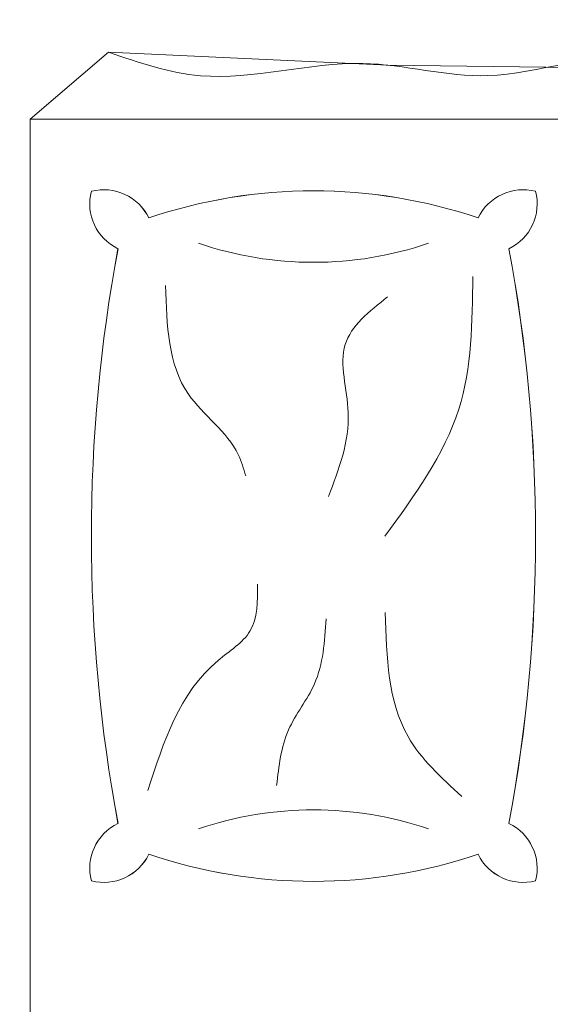
# Model space of a CAD drawing. Units: inches. Extents: x 2083 to 3317, y 1141 to 2115.
# Tile 7 of 256: x 2241 to 2260, y 1327 to 1361. Entities that reach past the tile are written whole.
import ezdxf

# ---------------------------------------------------------------- set-up
doc = ezdxf.new("R2010")
doc.units = ezdxf.units.IN
for name, color, linetype, lineweight in [('A-ANNO-DIMS', 2, 'Continuous', 18), ('A-FURN', 8, 'Continuous', 18), ('www.cadblocksfree.com', 7, 'Continuous', 9)]:
    doc.layers.add(name, color=color, linetype=linetype, lineweight=lineweight)
doc.layers.add('A-WALL-PATT', color=251, linetype='Continuous', lineweight=13, true_color=0x636466)
doc.styles.get("Standard").update_dxf_attribs({"font": 'arial.ttf'})
doc.dimstyles.new('ISO-25', dxfattribs={"dimtxt": 12, "dimasz": 12, "dimexe": 1.25, "dimexo": 0.625, "dimtad": 1, "dimlunit": 3, "dimtxsty": 'Standard', "dimcen": 2.5, "dimadec": 0, "dimazin": 0, "dimtfac": 1, "dimtmove": 0, "dimatfit": 3, "dimfxl": 1, "dimarcsym": 0})

# ---------------------------------------------------------------- blocks, each defined once
blk = doc.blocks.new('bed')
at = {"layer": 'www.cadblocksfree.com', "ltscale": 0.2}
blk.add_line((3426.379, 1470.154), (3428.883, 1467.22), dxfattribs=at)
blk.add_lwpolyline([(3426.379, 1449.413), (3426.379, 1470.154), (3363.387, 1470.154), (3363.387, 1447.076)], dxfattribs=at)
for centre, radius, start, end in [((3398.298, 1466.054), 1.87, 25.7901, 104.4834), ((3423.206, 1466.054), 1.87, 75.5166, 154.2099), ((3399.641, 1467.396), 1.87, 165.5166, 244.2099), ((3410.752, 1409.187), 58.677, 79.42346, 100.57654), ((3421.863, 1467.396), 1.87, 295.7901, 14.4834), ((3417.027, 1459.547), 19.215, 161.2852, 198.7148), ((3404.477, 1459.547), 19.215, 341.2852, 18.7148), ((3387.154, 1459.547), 13.338, 341.1598, 18.8402), ((3434.35, 1459.547), 13.338, 161.1598, 198.8402), ((3399.641, 1451.698), 1.87, 115.7901, 194.4834), ((3421.863, 1451.698), 1.87, 345.5166, 64.2099), ((3398.298, 1453.041), 1.87, 255.5166, 334.2099), ((3410.752, 1509.907), 58.677, 259.42346, 280.57654), ((3423.206, 1453.041), 1.87, 205.7901, 284.4834)]:
    blk.add_arc(centre, radius, start, end, dxfattribs=at)
for points, knots in [([(3428.883, 1467.22), (3428.494, 1466.08), (3427.438, 1462.983), (3429.036, 1458.154), (3427.377, 1452.621), (3429.083, 1448.872), (3428.374, 1446.522), (3428.273, 1446.192)], [0, 0, 0, 0, 0.0901802, 0.2449351, 0.3646438, 0.5132331, 0.5378548, 0.5378548, 0.5378548, 0.5378548]), ([(3401.221, 1465.744), (3403.047, 1465.161), (3405.408, 1464.407), (3407.088, 1461.635), (3408.312, 1461.638), (3408.953, 1461.64)], [0, 0, 0, 0, 5.530688, 7.154877, 8.940839, 8.940839, 8.940839, 8.940839]), ([(3420.141, 1465.083), (3418.661, 1465.041), (3416.141, 1464.969), (3414.502, 1462.52), (3413.283, 1462.165), (3413.011, 1462.086)], [0, 0, 0, 0, 4.163459, 7.093919, 7.934624, 7.934624, 7.934624, 7.934624]), ([(3401.408, 1460.927), (3402.126, 1460.846), (3403.512, 1460.689), (3405.283, 1459.224), (3406.806, 1459.127), (3407.654, 1459.073)], [0, 0, 0, 0, 2.127543, 4.10272, 6.58647, 6.58647, 6.58647, 6.58647]), ([(3419.716, 1456.774), (3419.174, 1457.459), (3418.052, 1458.876), (3415.084, 1457.893), (3413.26, 1458.594), (3412.241, 1458.985)], [0, 0, 0, 0, 2.388143, 4.935423, 8.166198, 8.166198, 8.166198, 8.166198]), ([(3400.996, 1453.995), (3401.698, 1454.761), (3403.498, 1456.726), (3406.222, 1456.811), (3407.884, 1456.863)], [0, 0, 0, 0, 3.013696, 7.735839, 7.735839, 7.735839, 7.735839]), ([(3420.479, 1453.579), (3418.77, 1453.599), (3415.179, 1453.639), (3412.269, 1455.762), (3410.745, 1456.874)], [0, 0, 0, 0, 5.002087, 10.507046, 10.507046, 10.507046, 10.507046])]:
    blk.add_open_spline(points, degree=3, knots=knots, dxfattribs=at)
blk = doc.blocks.new('*D22')
at = {"layer": 'A-ANNO-DIMS', "color": 0, "lineweight": -2, "transparency": 16777216}
for p, q in [((2235.96, 1362.739), (2235.96, 1376.309)), ((2322.26, 1362.739), (2322.26, 1376.309)), ((2235.96, 1375.059), (2083.007, 1375.059)), ((2310.26, 1375.059), (2247.96, 1375.059))]:
    blk.add_line(p, q, dxfattribs=at)
at = {"layer": 'A-ANNO-DIMS', "color": 0, "transparency": 16777216}
for points in [[(2247.96, 1377.059), (2247.96, 1373.059), (2235.96, 1375.059)], [(2310.26, 1377.059), (2310.26, 1373.059), (2322.26, 1375.059)]]:
    blk.add_solid(points, dxfattribs=at)
at = {"layer": 'Defpoints', "color": 0, "transparency": 16777216}
for p in [(2235.96, 1375.059), (2235.96, 1362.114), (2322.26, 1362.114)]:
    blk.add_point(p, dxfattribs=at)
at = {"layer": 'A-ANNO-DIMS', "color": 0, "transparency": 16777216, "insert": (2153.483, 1381.889), "char_height": 12, "attachment_point": 5}
blk.add_mtext('BED 7\'-2 1/2" TYP.', dxfattribs=at)

msp = doc.modelspace()

# ---------------------------------------------------------------- hatches: boundary and pattern name
at = {"layer": 'A-WALL-PATT'}
h = msp.add_hatch(color=256, dxfattribs=at)
h.dxf.hatch_style = 1
h.paths.add_polyline_path([(3126.96, 2020.761), (2748.96, 2020.761), (2604.96, 2020.761), (2226.96, 2020.761), (2226.96, 1702.761), (2466.96, 1702.761), (2466.96, 1582.761), (2418.96, 1582.761), (2418.96, 1477.761), (2226.96, 1477.761), (2226.96, 1263.261), (2544.96, 1263.261), (2544.96, 1411.761), (2604.96, 1411.761), (2685.96, 1411.761), (2685.96, 1420.761), (2604.96, 1420.761), (2604.96, 1573.761), (2604.96, 1702.761), (2604.96, 2011.761), (2748.96, 2011.761), (2748.96, 1702.761), (2862.96, 1702.761), (2862.96, 1621.761), (2871.96, 1621.761), (2871.96, 1702.761), (2883.96, 1702.761), (2883.96, 1706.939, -0.026459), (2883.96, 1711.761), (2757.96, 1711.761), (2757.96, 1807.761), (2787.96, 1807.761), (2787.96, 1812.261), (2757.96, 1812.261), (2757.96, 2011.761), (2877.96, 2011.761), (2877.96, 1812.261), (2847.96, 1812.261), (2847.96, 1807.761), (2889.836, 1807.761), (2889.836, 1812.261), (2882.46, 1812.261), (2882.46, 2011.761), (3117.96, 2011.761), (3117.96, 1812.261), (2937.836, 1812.261), (2937.836, 1807.761), (2995.71, 1807.761), (2995.71, 1796.118), (3000.21, 1796.118), (3000.21, 1807.761), (3117.96, 1807.761), (3117.96, 1711.761), (3000.21, 1711.761), (3000.21, 1760.118), (2998.573, 1760.118, -0.020711), (2995.71, 1760.118), (2995.71, 1711.761), (2931.96, 1711.761), (2931.96, 1702.761), (3126.96, 1702.761)])
h.paths.add_polyline_path([(2471.46, 2011.761), (2471.46, 1810.011), (2462.717, 1810.011), (2462.717, 1805.511), (2505.96, 1805.511), (2505.96, 1810.011), (2475.96, 1810.011), (2475.96, 2011.761), (2595.96, 2011.761), (2595.96, 1810.011), (2565.96, 1810.011), (2565.96, 1805.511), (2595.96, 1805.511), (2595.96, 1711.761), (2235.96, 1711.761), (2235.96, 1805.511), (2353.71, 1805.511), (2353.71, 1796.054), (2358.21, 1796.054), (2358.21, 1805.511), (2414.717, 1805.511), (2414.717, 1810.011), (2235.96, 1810.011), (2235.96, 2011.761)], flags=16)
h.paths.add_polyline_path([(2270.205, 1994.61), (2270.205, 1970.61), (2246.205, 1970.61), (2246.205, 1994.61)], flags=0)
edge = h.paths.add_edge_path(flags=0)
edge.add_ellipse((2332.027, 1899.798), major_axis=(-3.043, 3.043), ratio=0.168252, start_angle=-161.3322, end_angle=-156.3071, ccw=False)
edge.add_ellipse((2333.082, 1898.744), major_axis=(-1.055, 1.055), ratio=0.453532, start_angle=-123.371, end_angle=-94.1591)
edge = h.paths.add_edge_path(flags=0)
edge.add_ellipse((2332.027, 1968.876), major_axis=(3.043, 3.043), ratio=0.168252, start_angle=18.6678, end_angle=23.6929)
edge.add_spline(control_points=[(2332.926, 1970.691), (2332.227, 1970.336), (2330.894, 1969.659), (2328.413, 1970.932), (2327.204, 1967.749), (2324.71, 1969.956), (2322.533, 1967.012), (2320.013, 1971.296), (2317.68, 1968.158), (2316.041, 1967.102), (2315.427, 1966.81)], knot_values=[0, 0, 0, 0, 2.267059, 4.324559, 6.685584, 8.878641, 11.121502, 14.300359, 17.755284, 19.732645, 19.732645, 19.732645, 19.732645], degree=3, periodic=0)
edge.add_ellipse((2332.027, 1968.876), major_axis=(3.043, 3.043), ratio=0.168252, start_angle=18.6678, end_angle=23.6929, ccw=False)
edge.add_ellipse((2333.082, 1969.931), major_axis=(1.055, 1.055), ratio=0.453532, start_angle=56.629, end_angle=85.8409, ccw=False)
edge = h.paths.add_edge_path(flags=0)
edge.add_spline(control_points=[(2296.428, 1967.988), (2293.628, 1965.336), (2287.704, 1959.727), (2299.744, 1949.996), (2294.533, 1935.669), (2290.573, 1920.604), (2293.394, 1909.974), (2296.185, 1904.967)], knot_values=[0.099185, 0.099185, 0.099185, 0.099185, 0.345301, 0.619822, 0.982653, 1.386093, 1.810555, 1.810555, 1.810555, 1.810555], degree=3, periodic=0)
edge.add_spline(control_points=[(2296.185, 1904.967), (2297.384, 1902.619), (2298.001, 1901.949), (2298.553, 1901.468)], knot_values=[0.006246, 0.006246, 0.006246, 0.006246, 0.055476, 0.055476, 0.055476, 0.055476], degree=3, periodic=0)
edge.add_spline(control_points=[(2298.553, 1901.468), (2297.259, 1900.923), (2295.225, 1900.232), (2293.06, 1900.614), (2292.101, 1900.788), (2292.09, 1900.791)], knot_values=[0.312835, 0.312835, 0.312835, 0.312835, 0.40178, 0.474987, 0.475903, 0.475903, 0.475903, 0.475903], degree=3, periodic=0)
edge.add_arc((2292.794, 1904.664), 3.937, 215.4209, 259.6982, ccw=False)
edge.add_spline(control_points=[(2289.585, 1902.382), (2289.477, 1902.535), (2289.368, 1902.688), (2289.261, 1902.841)], knot_values=[0.102872, 0.102872, 0.102872, 0.102872, 0.116896, 0.116896, 0.116896, 0.116896], degree=3, periodic=0)
edge.add_spline(control_points=[(2289.261, 1902.841), (2288.687, 1902.55), (2287.64, 1902.02), (2285.881, 1901.874), (2283.853, 1901.504), (2281.72, 1899.711), (2278.467, 1899.493), (2276.157, 1901.883), (2272.259, 1899.804), (2267.778, 1901.843), (2262.244, 1900.184), (2257.415, 1901.782), (2254.318, 1900.726), (2253.178, 1900.337)], knot_values=[0, 0, 0, 0, 1.907977, 3.477176, 5.261074, 7.972851, 11.680248, 13.717921, 16.939592, 22.789562, 27.502503, 33.595215, 37.145618, 37.145618, 37.145618, 37.145618], degree=3, periodic=0)
edge.add_line((2253.178, 1900.337), (2250.244, 1902.841))
edge.add_line((2250.244, 1902.841), (2250.244, 1965.833))
edge.add_line((2250.244, 1965.833), (2253.178, 1968.337))
edge.add_spline(control_points=[(2253.178, 1968.337), (2254.318, 1967.948), (2257.415, 1966.892), (2262.244, 1968.49), (2267.778, 1966.831), (2271.527, 1968.537), (2273.876, 1967.828), (2274.207, 1967.728)], knot_values=[0, 0, 0, 0, 0.09018, 0.244935, 0.364644, 0.513233, 0.537855, 0.537855, 0.537855, 0.537855], degree=3, periodic=0)
edge.add_arc((2274.353, 1963.793), 3.937, 72.0511, 92.1279, ccw=False)
edge.add_arc((2281.297, 1985.23), 18.596, 252.0511, 288.5657)
edge.add_arc((2292.317, 1956.029), 12.646, 71.0268, 113.7782, ccw=False)
edge = h.paths.add_edge_path(flags=0)
edge.add_spline(control_points=[(2274.899, 1951.856), (2275.066, 1951.617), (2275.233, 1951.377), (2275.398, 1951.136)], knot_values=[1.409916, 1.409916, 1.409916, 1.409916, 1.43159, 1.43159, 1.43159, 1.43159], degree=3, periodic=0)
edge.add_spline(control_points=[(2275.398, 1951.136), (2275.792, 1950.562), (2276.179, 1949.984), (2276.546, 1949.397)], knot_values=[1.358238, 1.358238, 1.358238, 1.358238, 1.409916, 1.409916, 1.409916, 1.409916], degree=3, periodic=0)
edge.add_line((2276.546, 1949.397), (2277.437, 1947.862))
edge.add_spline(control_points=[(2277.437, 1947.862), (2276.304, 1945.673), (2274.64, 1942.427), (2274.632, 1938.094), (2272.799, 1930.852), (2274.356, 1943.897), (2275.948, 1947.923), (2276.546, 1949.397)], knot_values=[0.005632, 0.005632, 0.005632, 0.005632, 0.186014, 0.266002, 0.357087, 0.59639, 0.739732, 0.739732, 0.739732, 0.739732], degree=3, periodic=0)
edge.add_spline(control_points=[(2276.546, 1949.397), (2276.179, 1949.984), (2275.792, 1950.562), (2275.398, 1951.136)], knot_values=[1.358238, 1.358238, 1.358238, 1.358238, 1.409916, 1.409916, 1.409916, 1.409916], degree=3, periodic=0)
edge.add_spline(control_points=[(2275.398, 1951.136), (2274.943, 1950.08), (2274.208, 1948.025), (2273.935, 1944.851), (2272.469, 1937.627), (2273.466, 1945.696), (2274.701, 1951.059), (2274.899, 1951.856)], knot_values=[0.104364, 0.104364, 0.104364, 0.104364, 0.189636, 0.269624, 0.36071, 0.600013, 0.644622, 0.644622, 0.644622, 0.644622], degree=3, periodic=0)
h.paths.add_polyline_path([(2269.168, 1963.128, -0.357527), (2268.171, 1960.976, -0.092561), (2268.171, 1939.436, -0.357527), (2269.168, 1937.285, -0.357527), (2267.016, 1938.282, -0.164785), (2254.686, 1938.282, -0.357527), (2252.534, 1937.285, -0.357527), (2253.531, 1939.436, -0.092561), (2253.531, 1960.976, -0.357527), (2252.534, 1963.128, -0.357527), (2254.686, 1962.131, -0.164785), (2267.016, 1962.131, -0.357527)], flags=0)
h.paths.add_polyline_path([(2248.874, 1967.802), (2248.874, 1957.028), (2249.458, 1957.028), (2249.458, 1911.647), (2248.874, 1911.647), (2248.874, 1900.873), (2246.512, 1900.873, 0.197327), (2244.15, 1902.457), (2244.15, 1966.218, 0.197327), (2246.512, 1967.802)], flags=0)
h.paths.add_polyline_path([(2269.168, 1931.389, -0.357527), (2268.171, 1929.238, -0.092561), (2268.171, 1907.698, -0.357527), (2269.168, 1905.547, -0.357527), (2267.016, 1906.544, -0.164785), (2254.686, 1906.544, -0.357527), (2252.534, 1905.547, -0.357527), (2253.531, 1907.698, -0.092561), (2253.531, 1929.238, -0.357527), (2252.534, 1931.389, -0.357527), (2254.686, 1930.392, -0.164785), (2267.016, 1930.392, -0.357527)], flags=0)
edge = h.paths.add_edge_path(flags=0)
edge.add_spline(control_points=[(2276.197, 1906.724), (2276.168, 1909.029), (2276.114, 1913.372), (2270.598, 1924.925), (2273.905, 1919.013), (2275.922, 1916.262), (2275.475, 1912.402), (2277.258, 1910.381), (2276.696, 1908.225), (2276.646, 1906.813), (2276.618, 1906.008)], knot_values=[0, 0, 0, 0, 8.61026, 16.221274, 18.843057, 23.804898, 27.440828, 29.356102, 31.203478, 33.650687, 33.650687, 33.650687, 33.650687], degree=3, periodic=0)
edge.add_spline(control_points=[(2276.618, 1906.008), (2276.623, 1905.624), (2276.498, 1904.629), (2275.442, 1903.855), (2274.937, 1903.08), (2274.859, 1902.841)], knot_values=[0.156488, 0.156488, 0.156488, 0.156488, 0.184398, 0.231376, 0.250598, 0.250598, 0.250598, 0.250598], degree=3, periodic=0)
edge.add_line((2274.859, 1902.841), (2276.506, 1902.841))
edge.add_spline(control_points=[(2276.506, 1902.841), (2276.788, 1903.085), (2277.665, 1904.125), (2278.25, 1904.341), (2277.654, 1908.527), (2278.156, 1906.228), (2278.1, 1905.286), (2278.847, 1904.069), (2277.857, 1903.415), (2277.874, 1902.991), (2277.904, 1902.841)], knot_values=[0.059574, 0.059574, 0.059574, 0.059574, 0.080753, 0.103741, 0.16972, 0.176036, 0.207137, 0.240474, 0.262341, 0.27366, 0.27366, 0.27366, 0.27366], degree=3, periodic=0)
edge.add_line((2277.904, 1902.841), (2280.03, 1902.841))
edge.add_spline(control_points=[(2280.03, 1902.841), (2279.888, 1903.088), (2279.499, 1903.982), (2280.152, 1905.939), (2278.104, 1909.658), (2279.762, 1907.185), (2280.328, 1904.875), (2280.485, 1903.49), (2281.463, 1903.249), (2281.758, 1902.936), (2281.834, 1902.841)], knot_values=[0.013856, 0.013856, 0.013856, 0.013856, 0.034874, 0.088867, 0.107879, 0.126738, 0.158714, 0.193757, 0.217487, 0.226722, 0.226722, 0.226722, 0.226722], degree=3, periodic=0)
edge.add_spline(control_points=[(2281.834, 1902.841), (2281.788, 1902.827), (2281.647, 1902.783), (2281.396, 1902.859), (2281.088, 1902.985), (2280.721, 1903.061), (2280.333, 1903.026), (2280.125, 1902.899), (2280.03, 1902.841)], knot_values=[0, 0, 0, 0, 0.14413, 0.435517, 0.749276, 1.153046, 1.548371, 1.878348, 1.878348, 1.878348, 1.878348], degree=3, periodic=0)
edge.add_line((2280.03, 1902.841), (2277.904, 1902.841))
edge.add_spline(control_points=[(2277.904, 1902.841), (2277.893, 1902.796), (2277.865, 1902.68), (2277.607, 1902.687), (2277.274, 1902.801), (2276.838, 1902.62), (2276.584, 1902.789), (2276.506, 1902.841)], knot_values=[0, 0, 0, 0, 0.127189, 0.326199, 0.628009, 1.24357, 1.515331, 1.515331, 1.515331, 1.515331], degree=3, periodic=0)
edge.add_line((2276.506, 1902.841), (2274.859, 1902.841))
edge.add_spline(control_points=[(2274.859, 1902.841), (2274.814, 1902.899), (2274.725, 1903.013), (2274.493, 1903.119), (2274.244, 1902.961), (2273.937, 1903.185), (2273.614, 1902.983), (2273.408, 1902.883), (2273.322, 1902.841)], knot_values=[0, 0, 0, 0, 0.21843, 0.436957, 0.687977, 0.990379, 1.398396, 1.69185, 1.69185, 1.69185, 1.69185], degree=3, periodic=0)
edge.add_spline(control_points=[(2273.322, 1902.841), (2273.617, 1903.446), (2274.274, 1904.538), (2276.027, 1904.574), (2276.207, 1906.584), (2276.197, 1906.724)], knot_values=[0.012227, 0.012227, 0.012227, 0.012227, 0.059472, 0.106218, 0.134458, 0.134458, 0.134458, 0.134458], degree=3, periodic=0)
h.paths.add_polyline_path([(2270.776, 1897.79), (2270.776, 1873.79), (2246.776, 1873.79), (2246.776, 1897.79)], flags=0)
h.paths.add_polyline_path([(2353.71, 1760.005), (2353.71, 1760.054), (2358.21, 1760.054, -0.033729)], flags=0)
h.paths.add_polyline_path([(2321.819, 1737.529), (2341.995, 1737.529, -0.414214), (2343.203, 1736.321), (2343.203, 1721.021, -0.414214), (2341.995, 1719.813), (2321.819, 1719.813, -0.414214), (2320.611, 1721.021), (2320.611, 1736.321, -0.414214)], flags=0)
h.paths.add_polyline_path([(2324.235, 1736.321), (2339.579, 1736.321, -0.414214), (2341.995, 1733.905), (2341.995, 1725.45, -0.414214), (2339.579, 1723.034), (2333.681, 1723.034), (2333.845, 1722.045, -0.870646), (2335.425, 1721.826, -0.767327), (2333.923, 1721.423), (2331.291, 1721.423, -0.767327), (2329.788, 1721.826, -0.870646), (2331.368, 1722.045), (2331.533, 1723.034), (2324.235, 1723.034, -0.414214), (2321.819, 1725.45), (2321.819, 1733.905, -0.414214)], flags=0)
h.paths.add_polyline_path([(2570.484, 1928.615), (2589.684, 1928.615), (2590.169, 1928.615), (2590.169, 1904.993), (2570.484, 1904.993)], flags=0)
h.paths.add_polyline_path([(2574.447, 1927.264, -1), (2572.829, 1927.264, -1)], flags=0)
h.paths.add_polyline_path([(2573.09, 1926.941), (2573.925, 1927.776), (2574.148, 1927.553), (2573.313, 1926.718)], flags=0)
h.paths.add_polyline_path([(2578.779, 1919.73, -1), (2571.592, 1919.73, -1)], flags=0)
h.paths.add_polyline_path([(2578.385, 1919.73, -1), (2571.985, 1919.73, -1)], flags=0)
h.paths.add_polyline_path([(2331.596, 1729.476, -1), (2333.618, 1729.476, -1)], flags=0)
h.paths.add_polyline_path([(2578.034, 1927.264, -1), (2576.416, 1927.264, -1)], flags=0)
h.paths.add_polyline_path([(2576.689, 1927.531), (2576.912, 1927.754), (2577.747, 1926.919), (2577.524, 1926.696)], flags=0)
h.paths.add_polyline_path([(2578.139, 1909.86, -1), (2572.232, 1909.86, -1)], flags=0)
h.paths.add_polyline_path([(2577.745, 1909.86, -1), (2572.625, 1909.86, -1)], flags=0)
h.paths.add_polyline_path([(2583.798, 1927.264, -1), (2582.179, 1927.264, -1)], flags=0)
h.paths.add_polyline_path([(2582.719, 1927.754), (2583.554, 1926.919), (2583.331, 1926.696), (2582.496, 1927.531)], flags=0)
h.paths.add_polyline_path([(2582.496, 1927.531), (2582.719, 1927.754), (2583.554, 1926.919), (2583.331, 1926.696)], flags=0)
h.paths.add_polyline_path([(2587.739, 1920.53, -1), (2581.832, 1920.53, -1)], flags=0)
h.paths.add_polyline_path([(2587.345, 1920.53, -1), (2582.225, 1920.53, -1)], flags=0)
h.paths.add_polyline_path([(2587.385, 1927.264, -1), (2585.766, 1927.264, -1)], flags=0)
h.paths.add_polyline_path([(2586.082, 1926.98), (2586.917, 1927.815), (2587.14, 1927.593), (2586.305, 1926.758)], flags=0)
h.paths.add_polyline_path([(2588.379, 1910.66, -1), (2581.192, 1910.66, -1)], flags=0)
h.paths.add_polyline_path([(2587.985, 1910.66, -1), (2581.585, 1910.66, -1)], flags=0)
h.paths.add_polyline_path([(2417.168, 1729.478), (2437.344, 1729.478, -0.414214), (2438.552, 1728.27), (2438.552, 1712.969, -0.414214), (2437.344, 1711.761), (2417.168, 1711.761, -0.414214), (2415.96, 1712.969), (2415.96, 1728.27, -0.414214)], flags=0)
h.paths.add_polyline_path([(2419.584, 1728.27), (2434.928, 1728.27, -0.414214), (2437.344, 1725.854), (2437.344, 1717.398, -0.414214), (2434.928, 1714.983), (2429.029, 1714.983), (2429.194, 1713.994, -0.870646), (2430.774, 1713.775, -0.767327), (2429.271, 1713.372), (2426.64, 1713.372, -0.767327), (2425.137, 1713.775, -0.870646), (2426.717, 1713.994), (2426.882, 1714.983), (2419.584, 1714.983, -0.414214), (2417.168, 1717.398), (2417.168, 1725.854, -0.414214)], flags=0)
h.paths.add_polyline_path([(2419.584, 1728.27), (2434.928, 1728.27, -0.414214), (2437.344, 1725.854), (2437.344, 1717.398, -0.414214), (2434.928, 1714.983), (2429.029, 1714.983), (2428.358, 1719.009), (2427.553, 1719.009), (2426.882, 1714.983), (2419.584, 1714.983, -0.414214), (2417.168, 1717.398), (2417.168, 1725.854, -0.414214)], flags=0)
h.paths.add_polyline_path([(2426.944, 1721.425, -1), (2428.967, 1721.425, -1)], flags=0)
h.paths.add_polyline_path([(2475.96, 1702.761), (2595.96, 1702.761), (2595.96, 1582.761), (2475.96, 1582.761)], flags=16)
h.paths.add_polyline_path([(2427.96, 1573.761), (2595.96, 1573.761), (2595.96, 1468.761), (2595.96, 1420.761), (2384.46, 1420.761), (2384.46, 1468.761), (2427.96, 1468.761)], flags=16)
h.paths.add_polyline_path([(2379.96, 1468.761), (2379.96, 1420.761), (2235.96, 1420.761), (2235.96, 1468.761)], flags=16)
h.paths.add_polyline_path([(2317.816, 1466.696), (2337.992, 1466.696, -0.414214), (2339.2, 1465.488), (2339.2, 1450.187, -0.414214), (2337.992, 1448.979), (2317.816, 1448.979, -0.414214), (2316.608, 1450.187), (2316.608, 1465.488, -0.414214)], flags=0)
h.paths.add_polyline_path([(2320.232, 1465.488), (2335.576, 1465.488, -0.414214), (2337.992, 1463.072), (2337.992, 1454.616, -0.414214), (2335.576, 1452.2), (2329.677, 1452.2), (2329.842, 1451.212, -0.870646), (2331.422, 1450.992, -0.767327), (2329.92, 1450.59), (2327.288, 1450.59, -0.767327), (2325.785, 1450.992, -0.870646), (2327.365, 1451.212), (2327.53, 1452.2), (2320.232, 1452.2, -0.414214), (2317.816, 1454.616), (2317.816, 1463.072, -0.414214)], flags=0)
h.paths.add_polyline_path([(2320.232, 1465.488), (2335.576, 1465.488, -0.414214), (2337.992, 1463.072), (2337.992, 1454.616, -0.414214), (2335.576, 1452.2), (2329.677, 1452.2), (2329.006, 1456.227), (2328.201, 1456.227), (2327.53, 1452.2), (2320.232, 1452.2, -0.414214), (2317.816, 1454.616), (2317.816, 1463.072, -0.414214)], flags=0)
h.paths.add_polyline_path([(2327.593, 1458.643, -1), (2329.615, 1458.643, -1)], flags=0)
h.paths.add_polyline_path([(2244.412, 1433.34), (2241.921, 1433.34, -0.414214), (2240.018, 1435.244), (2240.018, 1440.953, -0.414211), (2241.921, 1442.856), (2244.412, 1442.856, -1.976472)], flags=0)
h.paths.add_polyline_path([(2245.357, 1434.398, -0.414214), (2245.357, 1441.799, -2.144098)], flags=0)
h.paths.add_polyline_path([(2535.96, 1416.261), (2535.96, 1272.261), (2235.96, 1272.261), (2235.96, 1416.261)], flags=16)
h.paths.add_polyline_path([(2260.12, 1384.293), (2260.12, 1362.039), (2237.865, 1362.039), (2237.865, 1384.293)], flags=0)
edge = h.paths.add_edge_path(flags=0)
edge.add_line((2318.252, 1362.093), (2318.146, 1362.001))
edge.add_ellipse((2317.445, 1360.431), major_axis=(2.822, 2.822), ratio=0.168252, start_angle=18.6678, end_angle=20.9481, ccw=False)
edge.add_ellipse((2318.423, 1361.409), major_axis=(0.978, 0.978), ratio=0.453532, start_angle=56.629, end_angle=70.2262, ccw=False)
edge = h.paths.add_edge_path(flags=0)
edge.add_line((2319.107, 1295.571), (2319.015, 1295.677))
edge.add_ellipse((2317.445, 1296.378), major_axis=(-2.822, 2.822), ratio=0.168252, start_angle=-161.3322, end_angle=-159.0519, ccw=False)
edge.add_ellipse((2318.423, 1295.4), major_axis=(-0.978, 0.978), ratio=0.453532, start_angle=-123.371, end_angle=-109.7738)
edge = h.paths.add_edge_path(flags=0)
edge.add_spline(control_points=[(2284.21, 1301.17), (2284.581, 1300.445), (2284.891, 1299.892), (2285.16, 1299.461)], knot_values=[0.039066, 0.039066, 0.039066, 0.039066, 0.055476, 0.055476, 0.055476, 0.055476], degree=3, periodic=0)
edge.add_line((2285.16, 1299.461), (2284.21, 1301.17))
edge = h.paths.add_edge_path(flags=0)
edge.add_line((2280.412, 1297.298), (2283.37, 1297.036))
edge.add_line((2283.37, 1297.036), (2286.406, 1297.926))
edge.add_spline(control_points=[(2286.406, 1297.926), (2285.305, 1297.463), (2284.345, 1297.129), (2283.37, 1297.036)], knot_values=[0.394369, 0.394369, 0.394369, 0.394369, 0.475903, 0.475903, 0.475903, 0.475903], degree=3, periodic=0)
edge.add_spline(control_points=[(2283.37, 1297.036), (2283.281, 1297.028), (2282.316, 1296.957), (2281.313, 1297.134), (2280.423, 1297.296), (2280.412, 1297.298)], knot_values=[0.312835, 0.312835, 0.312835, 0.312835, 0.320246, 0.393453, 0.394369, 0.394369, 0.394369, 0.394369], degree=3, periodic=0)
edge = h.paths.add_edge_path(flags=0)
edge.add_line((2284.436, 1359.607), (2280.446, 1355.328))
edge.add_line((2280.446, 1355.328), (2279.58, 1351.018))
edge.add_line((2279.58, 1351.018), (2282.413, 1346.58))
edge.add_spline(control_points=[(2282.413, 1346.58), (2283.153, 1345.589), (2284.253, 1344.029), (2284.801, 1342.387), (2284.935, 1341.806)], knot_values=[1.240098, 1.240098, 1.240098, 1.240098, 1.332892, 1.382712, 1.382712, 1.382712, 1.382712], degree=3, periodic=0)
edge.add_spline(control_points=[(2284.935, 1341.806), (2285.319, 1340.141), (2285.233, 1338.409), (2284.91, 1336.654)], knot_values=[1.097484, 1.097484, 1.097484, 1.097484, 1.240098, 1.240098, 1.240098, 1.240098], degree=3, periodic=0)
edge.add_spline(control_points=[(2284.91, 1336.654), (2284.587, 1334.899), (2284.027, 1333.12), (2283.463, 1331.361)], knot_values=[0.95487, 0.95487, 0.95487, 0.95487, 1.097484, 1.097484, 1.097484, 1.097484], degree=3, periodic=0)
edge.add_line((2283.463, 1331.361), (2281.89, 1326.153))
edge.add_line((2281.89, 1326.153), (2280.756, 1321.056))
edge.add_line((2280.756, 1321.056), (2280.299, 1316.002))
edge.add_line((2280.299, 1316.002), (2280.716, 1310.95))
edge.add_line((2280.716, 1310.95), (2282.028, 1305.972))
edge.add_line((2282.028, 1305.972), (2284.21, 1301.17))
edge.add_spline(control_points=[(2284.21, 1301.17), (2283.341, 1302.73), (2282.612, 1304.336), (2282.028, 1305.972)], knot_values=[0.099185, 0.099185, 0.099185, 0.099185, 0.241799, 0.241799, 0.241799, 0.241799], degree=3, periodic=0)
edge.add_spline(control_points=[(2282.028, 1305.972), (2281.444, 1307.608), (2281.005, 1309.273), (2280.716, 1310.95)], knot_values=[0.241799, 0.241799, 0.241799, 0.241799, 0.384413, 0.384413, 0.384413, 0.384413], degree=3, periodic=0)
edge.add_spline(control_points=[(2280.716, 1310.95), (2280.433, 1312.588), (2280.289, 1314.277), (2280.299, 1315.962), (2280.299, 1316.002)], knot_values=[0.384413, 0.384413, 0.384413, 0.384413, 0.523647, 0.527028, 0.527028, 0.527028, 0.527028], degree=3, periodic=0)
edge.add_spline(control_points=[(2280.299, 1316.002), (2280.312, 1317.687), (2280.478, 1319.368), (2280.756, 1321.056)], knot_values=[0.527028, 0.527028, 0.527028, 0.527028, 0.669642, 0.669642, 0.669642, 0.669642], degree=3, periodic=0)
edge.add_spline(control_points=[(2280.756, 1321.056), (2281.035, 1322.744), (2281.426, 1324.44), (2281.89, 1326.153)], knot_values=[0.669642, 0.669642, 0.669642, 0.669642, 0.812256, 0.812256, 0.812256, 0.812256], degree=3, periodic=0)
edge.add_spline(control_points=[(2281.89, 1326.153), (2282.264, 1327.533), (2282.788, 1329.262), (2283.353, 1331.018), (2283.463, 1331.361)], knot_values=[0.812256, 0.812256, 0.812256, 0.812256, 0.927087, 0.95487, 0.95487, 0.95487, 0.95487], degree=3, periodic=0)
edge.add_line((2283.463, 1331.361), (2284.91, 1336.654))
edge.add_line((2284.91, 1336.654), (2284.935, 1341.806))
edge.add_line((2284.935, 1341.806), (2282.413, 1346.58))
edge.add_spline(control_points=[(2282.413, 1346.58), (2281.275, 1348.104), (2280.078, 1349.57), (2279.58, 1351.018)], knot_values=[1.382712, 1.382712, 1.382712, 1.382712, 1.525326, 1.525326, 1.525326, 1.525326], degree=3, periodic=0)
edge.add_spline(control_points=[(2279.58, 1351.018), (2279.443, 1351.415), (2279.136, 1352.857), (2279.735, 1354.29), (2280.446, 1355.328)], knot_values=[1.525326, 1.525326, 1.525326, 1.525326, 1.564439, 1.667941, 1.667941, 1.667941, 1.667941], degree=3, periodic=0)
edge.add_spline(control_points=[(2280.446, 1355.328), (2281.426, 1356.758), (2282.931, 1358.183), (2284.436, 1359.607)], knot_values=[1.667941, 1.667941, 1.667941, 1.667941, 1.810555, 1.810555, 1.810555, 1.810555], degree=3, periodic=0)
edge.add_arc((2280.623, 1348.518), 11.726, 71.0268, 113.7782)
edge.add_arc((2270.405, 1375.595), 17.244, 252.0511, 288.5657, ccw=False)
edge.add_arc((2263.966, 1355.718), 3.651, 72.0511, 92.1279)
edge.add_arc((2263.966, 1355.718), 3.651, 92.1279, 177.9851)
edge.add_spline(control_points=[(2260.318, 1355.846), (2260.26, 1354.221), (2260.551, 1350.187), (2262.999, 1346.766), (2264.473, 1344.649)], knot_values=[1.43159, 1.43159, 1.43159, 1.43159, 1.564144, 1.770695, 1.770695, 1.770695, 1.770695], degree=3, periodic=0)
edge.add_line((2264.473, 1344.649), (2264.936, 1343.983))
edge.add_spline(control_points=[(2263.801, 1340.248), (2263.843, 1340.514), (2264.067, 1341.756), (2264.513, 1343.002), (2264.935, 1343.981)], knot_values=[0.53657, 0.53657, 0.53657, 0.53657, 0.559349, 0.644622, 0.644622, 0.644622, 0.644622], degree=3, periodic=0)
edge.add_spline(control_points=[(2264.935, 1343.981), (2265.118, 1343.715), (2265.299, 1343.448), (2265.477, 1343.179)], knot_values=[1.384077, 1.384077, 1.384077, 1.384077, 1.409916, 1.409916, 1.409916, 1.409916], degree=3, periodic=0)
edge.add_spline(control_points=[(2265.477, 1343.179), (2265.655, 1342.911), (2265.829, 1342.641), (2265.999, 1342.369)], knot_values=[1.358238, 1.358238, 1.358238, 1.358238, 1.384077, 1.384077, 1.384077, 1.384077], degree=3, periodic=0)
edge.add_line((2265.999, 1342.369), (2266.826, 1340.946))
edge.add_spline(control_points=[(2266.826, 1340.946), (2268.894, 1337.09), (2271.398, 1325.843), (2270.516, 1310.569), (2275.919, 1301.861), (2277.79, 1299.199)], knot_values=[0.116896, 0.116896, 0.116896, 0.116896, 0.472987, 1.050969, 1.313793, 1.313793, 1.313793, 1.313793], degree=3, periodic=0)
edge.add_spline(control_points=[(2277.79, 1299.199), (2277.839, 1299.128), (2277.889, 1299.057), (2277.94, 1298.987)], knot_values=[0.109884, 0.109884, 0.109884, 0.109884, 0.116896, 0.116896, 0.116896, 0.116896], degree=3, periodic=0)
edge.add_line((2277.94, 1298.987), (2277.789, 1299.199))
edge.add_spline(control_points=[(2277.789, 1299.199), (2277.257, 1298.929), (2276.286, 1298.438), (2275.039, 1298.334), (2274.383, 1298.239), (2274.215, 1298.209)], knot_values=[33.12187, 33.12187, 33.12187, 33.12187, 35.029056, 36.598255, 37.144827, 37.144827, 37.144827, 37.144827], degree=3, periodic=0)
edge.add_line((2274.215, 1298.209), (2273.073, 1297.893))
edge.add_spline(control_points=[(2273.073, 1297.893), (2272.323, 1297.58), (2271.039, 1296.511), (2269.248, 1296.226), (2268.423, 1296.375)], knot_values=[26.532584, 26.532584, 26.532584, 26.532584, 29.198919, 31.839101, 31.839101, 31.839101, 31.839101], degree=3, periodic=0)
edge.add_line((2268.423, 1296.375), (2263.879, 1297.458))
edge.add_spline(control_points=[(2263.879, 1297.458), (2263.556, 1297.359), (2261.86, 1296.839), (2260.239, 1297.282), (2258.933, 1297.516)], knot_values=[15.919551, 15.919551, 15.919551, 15.919551, 16.939592, 21.226067, 21.226067, 21.226067, 21.226067], degree=3, periodic=0)
edge.add_line((2258.933, 1297.516), (2254.055, 1297.329))
edge.add_spline(control_points=[(2254.055, 1297.329), (2253.756, 1297.296), (2252.114, 1297.165), (2250.462, 1297.544), (2249.13, 1297.668)], knot_values=[5.306517, 5.306517, 5.306517, 5.306517, 6.276435, 10.613034, 10.613034, 10.613034, 10.613034], degree=3, periodic=0)
edge.add_line((2249.13, 1297.668), (2244.332, 1296.878))
edge.add_line((2244.332, 1296.878), (2241.611, 1299.199))
edge.add_line((2241.611, 1299.199), (2241.611, 1357.609))
edge.add_line((2241.611, 1357.609), (2244.332, 1359.931))
edge.add_line((2244.332, 1359.931), (2252.729, 1359.543))
edge.add_spline(control_points=[(2252.729, 1359.543), (2252.871, 1359.546), (2253.306, 1359.548), (2253.74, 1359.514), (2254.032, 1359.482)], knot_values=[0.233291, 0.233291, 0.233291, 0.233291, 0.244935, 0.268927, 0.268927, 0.268927, 0.268927], degree=3, periodic=0)
edge.add_line((2254.032, 1359.482), (2259.587, 1359.416))
edge.add_spline(control_points=[(2259.587, 1359.416), (2260.677, 1359.629), (2262.073, 1359.897), (2263.524, 1359.459), (2263.83, 1359.366)], knot_values=[0.422516, 0.422516, 0.422516, 0.422516, 0.513233, 0.537855, 0.537855, 0.537855, 0.537855], degree=3, periodic=0)
edge.add_arc((2263.966, 1355.718), 3.651, 72.0511, 92.1279, ccw=False)
edge.add_arc((2270.405, 1375.595), 17.244, 252.0511, 288.5657)
edge.add_arc((2280.623, 1348.518), 11.726, 71.0268, 113.7782, ccw=False)
h.paths.add_polyline_path([(2240.341, 1359.435), (2240.341, 1349.444), (2240.882, 1349.444), (2240.882, 1307.365), (2240.341, 1307.365), (2240.341, 1297.374), (2238.15, 1297.374, 0.197327), (2235.96, 1298.843), (2235.96, 1357.966, 0.197327), (2238.15, 1359.435)], flags=0)
h.paths.add_polyline_path([(2259.158, 1355.101, -0.357527), (2258.233, 1353.106, -0.092561), (2258.233, 1333.133, -0.357527), (2259.158, 1331.138, -0.357527), (2257.163, 1332.062, -0.164785), (2245.729, 1332.062, -0.357527), (2243.735, 1331.138, -0.357527), (2244.659, 1333.133, -0.092561), (2244.659, 1353.106, -0.357527), (2243.735, 1355.101, -0.357527), (2245.729, 1354.176, -0.164785), (2257.163, 1354.176, -0.357527)], flags=0)
edge = h.paths.add_edge_path(flags=0)
edge.add_line((2265.999, 1342.369), (2266.826, 1340.946))
edge.add_line((2266.826, 1340.946), (2265.308, 1337.814))
edge.add_line((2265.308, 1337.814), (2264.358, 1334.653))
edge.add_line((2264.358, 1334.653), (2264.262, 1333.8))
edge.add_spline(control_points=[(2264.262, 1333.8), (2264.208, 1333.187), (2264.162, 1332.366), (2264.007, 1331.414), (2263.969, 1331.202)], knot_values=[0.464444, 0.464444, 0.464444, 0.464444, 0.516691, 0.531608, 0.531608, 0.531608, 0.531608], degree=3, periodic=0)
edge.add_spline(control_points=[(2263.969, 1331.202), (2263.775, 1330.119), (2263.424, 1328.791), (2263.257, 1328.531), (2263.234, 1328.515)], knot_values=[0.372682, 0.372682, 0.372682, 0.372682, 0.44885, 0.464444, 0.464444, 0.464444, 0.464444], degree=3, periodic=0)
edge.add_spline(control_points=[(2263.234, 1328.515), (2263.096, 1328.42), (2263.131, 1329.301), (2263.275, 1330.616)], knot_values=[0.280919, 0.280919, 0.280919, 0.280919, 0.372682, 0.372682, 0.372682, 0.372682], degree=3, periodic=0)
edge.add_spline(control_points=[(2263.275, 1330.616), (2263.419, 1331.93), (2263.672, 1333.677), (2263.97, 1335.315)], knot_values=[0.189157, 0.189157, 0.189157, 0.189157, 0.280919, 0.280919, 0.280919, 0.280919], degree=3, periodic=0)
edge.add_spline(control_points=[(2263.97, 1335.315), (2264.1, 1336.032), (2264.419, 1337.622), (2264.755, 1338.864), (2264.947, 1339.491)], knot_values=[0.097394, 0.097394, 0.097394, 0.097394, 0.137578, 0.189157, 0.189157, 0.189157, 0.189157], degree=3, periodic=0)
edge.add_spline(control_points=[(2264.947, 1339.491), (2265.29, 1340.606), (2265.644, 1341.494), (2265.999, 1342.369)], knot_values=[0.005632, 0.005632, 0.005632, 0.005632, 0.097394, 0.097394, 0.097394, 0.097394], degree=3, periodic=0)
h.paths.add_polyline_path([(2259.158, 1325.671, -0.357527), (2258.233, 1323.676, -0.092561), (2258.233, 1303.703, -0.357527), (2259.158, 1301.708, -0.357527), (2257.163, 1302.633, -0.164785), (2245.729, 1302.633, -0.357527), (2243.735, 1301.708, -0.357527), (2244.659, 1303.703, -0.092561), (2244.659, 1323.676, -0.357527), (2243.735, 1325.671, -0.357527), (2245.729, 1324.747, -0.164785), (2257.163, 1324.747, -0.357527)], flags=0)
edge = h.paths.add_edge_path(flags=0)
edge.add_spline(control_points=[(2261.709, 1317.311), (2261.679, 1317.418), (2261.762, 1317.389), (2262.491, 1316.09), (2262.962, 1315.301)], knot_values=[14.955861, 14.955861, 14.955861, 14.955861, 16.221274, 18.694826, 18.694826, 18.694826, 18.694826], degree=3, periodic=0)
edge.add_spline(control_points=[(2262.962, 1315.301), (2262.99, 1315.254), (2263.702, 1314.067), (2264.349, 1313.127), (2264.73, 1312.164)], knot_values=[18.694826, 18.694826, 18.694826, 18.694826, 18.843057, 22.433791, 22.433791, 22.433791, 22.433791], degree=3, periodic=0)
edge.add_spline(control_points=[(2264.73, 1312.164), (2264.876, 1311.796), (2265.177, 1310.77), (2265.143, 1309.559), (2265.248, 1308.824)], knot_values=[22.433791, 22.433791, 22.433791, 22.433791, 23.804898, 26.172756, 26.172756, 26.172756, 26.172756], degree=3, periodic=0)
edge.add_line((2265.248, 1308.824), (2265.851, 1307.172))
edge.add_spline(control_points=[(2265.851, 1307.172), (2266.065, 1306.822), (2266.384, 1306.332), (2266.424, 1305.781), (2266.42, 1305.611)], knot_values=[28.062562, 28.062562, 28.062562, 28.062562, 29.356102, 29.911721, 29.911721, 29.911721, 29.911721], degree=3, periodic=0)
edge.add_spline(control_points=[(2266.42, 1305.611), (2266.416, 1305.433), (2266.394, 1305.25), (2266.365, 1305.066)], knot_values=[29.911721, 29.911721, 29.911721, 29.911721, 30.497837, 30.497837, 30.497837, 30.497837], degree=3, periodic=0)
edge.add_line((2266.365, 1305.066), (2266.066, 1302.136))
edge.add_spline(control_points=[(2266.066, 1302.136), (2266.071, 1301.78), (2265.998, 1301.2), (2265.663, 1300.759), (2265.509, 1300.586)], knot_values=[0.156488, 0.156488, 0.156488, 0.156488, 0.184398, 0.203543, 0.203543, 0.203543, 0.203543], degree=3, periodic=0)
edge.add_line((2265.509, 1300.586), (2264.435, 1299.199))
edge.add_line((2264.435, 1299.199), (2265.962, 1299.199))
edge.add_line((2265.962, 1299.199), (2267.336, 1301.175))
edge.add_line((2267.336, 1301.175), (2267.312, 1301.986))
edge.add_spline(control_points=[(2267.312, 1301.986), (2267.261, 1302.862), (2267.16, 1303.737), (2267.271, 1303.326)], knot_values=[0.126229, 0.126229, 0.126229, 0.126229, 0.166617, 0.166617, 0.166617, 0.166617], degree=3, periodic=0)
edge.add_spline(control_points=[(2267.271, 1303.326), (2267.28, 1303.294), (2267.31, 1303.175), (2267.373, 1302.884), (2267.406, 1302.683), (2267.418, 1302.601)], knot_values=[0.166617, 0.166617, 0.166617, 0.166617, 0.16972, 0.176036, 0.180765, 0.180765, 0.180765, 0.180765], degree=3, periodic=0)
edge.add_spline(control_points=[(2267.744, 1300.988), (2267.688, 1301.151), (2267.481, 1301.657), (2267.484, 1302.145), (2267.418, 1302.601)], knot_values=[0.180765, 0.180765, 0.180765, 0.180765, 0.193767, 0.220139, 0.220139, 0.220139, 0.220139], degree=3, periodic=0)
edge.add_line((2267.418, 1302.601), (2267.744, 1300.988))
edge.add_spline(control_points=[(2267.744, 1300.988), (2267.832, 1300.732), (2267.932, 1300.31), (2267.555, 1299.975), (2267.429, 1299.829)], knot_values=[0.220139, 0.220139, 0.220139, 0.220139, 0.240474, 0.25489, 0.25489, 0.25489, 0.25489], degree=3, periodic=0)
edge.add_line((2267.429, 1299.829), (2267.258, 1299.199))
edge.add_line((2267.258, 1299.199), (2269.23, 1299.199))
edge.add_spline(control_points=[(2269.23, 1299.199), (2269.099, 1299.429), (2268.843, 1300.016), (2269.012, 1300.916), (2268.947, 1301.661)], knot_values=[0.013856, 0.013856, 0.013856, 0.013856, 0.034874, 0.067073, 0.067073, 0.067073, 0.067073], degree=3, periodic=0)
edge.add_line((2268.947, 1301.661), (2268.432, 1303.603))
edge.add_spline(control_points=[(2268.432, 1303.603), (2268.176, 1304.192), (2267.596, 1305.251), (2268.041, 1304.623), (2268.251, 1304.282)], knot_values=[0.090155, 0.090155, 0.090155, 0.090155, 0.107879, 0.120289, 0.120289, 0.120289, 0.120289], degree=3, periodic=0)
edge.add_spline(control_points=[(2268.251, 1304.282), (2268.361, 1304.105), (2269.058, 1302.918), (2269.383, 1301.59), (2269.521, 1300.776), (2269.575, 1300.556)], knot_values=[0.120289, 0.120289, 0.120289, 0.120289, 0.126738, 0.158714, 0.173506, 0.173506, 0.173506, 0.173506], degree=3, periodic=0)
edge.add_line((2269.575, 1300.556), (2270.686, 1299.421))
edge.add_spline(control_points=[(2270.686, 1299.421), (2270.767, 1299.357), (2270.838, 1299.281), (2270.903, 1299.199)], knot_values=[0.21816, 0.21816, 0.21816, 0.21816, 0.226722, 0.226722, 0.226722, 0.226722], degree=3, periodic=0)
edge.add_line((2270.937, 1299.193), (2270.903, 1299.199))
edge.add_spline(control_points=[(2270.903, 1299.199), (2270.86, 1299.186), (2270.73, 1299.146), (2270.496, 1299.216), (2270.272, 1299.308), (2270.121, 1299.348), (2270.063, 1299.36)], knot_values=[0.939174, 0.939174, 0.939174, 0.939174, 1.083304, 1.374691, 1.68845, 1.878348, 1.878348, 1.878348, 1.878348], degree=3, periodic=0)
edge.add_line((2270.063, 1299.36), (2269.23, 1299.199))
edge.add_line((2269.23, 1299.199), (2267.258, 1299.199))
edge.add_spline(control_points=[(2267.258, 1299.199), (2267.248, 1299.157), (2267.223, 1299.05), (2266.984, 1299.057), (2266.809, 1299.116), (2266.677, 1299.109), (2266.637, 1299.105)], knot_values=[0.757665, 0.757665, 0.757665, 0.757665, 0.884854, 1.083864, 1.385675, 1.515331, 1.515331, 1.515331, 1.515331], degree=3, periodic=0)
edge.add_spline(control_points=[(2266.637, 1299.105), (2266.485, 1299.089), (2266.236, 1299.017), (2266.035, 1299.151), (2265.962, 1299.199)], knot_values=[0, 0, 0, 0, 0.485905, 0.757665, 0.757665, 0.757665, 0.757665], degree=3, periodic=0)
edge.add_line((2265.962, 1299.199), (2264.435, 1299.199))
edge.add_line((2264.435, 1299.199), (2263.858, 1299.367))
edge.add_spline(control_points=[(2263.858, 1299.367), (2263.819, 1299.371), (2263.78, 1299.386), (2263.74, 1299.402)], knot_values=[0.845925, 0.845925, 0.845925, 0.845925, 0.978627, 0.978627, 0.978627, 0.978627], degree=3, periodic=0)
edge.add_line((2263.722, 1299.396), (2263.01, 1299.199))
edge.add_spline(control_points=[(2263.01, 1299.199), (2263.246, 1299.683), (2263.506, 1300.128), (2263.873, 1300.408)], knot_values=[0.012227, 0.012227, 0.012227, 0.012227, 0.052971, 0.052971, 0.052971, 0.052971], degree=3, periodic=0)
edge.add_spline(control_points=[(2263.873, 1300.408), (2263.932, 1300.453), (2264.084, 1300.553), (2264.255, 1300.624), (2264.36, 1300.665)], knot_values=[0.052971, 0.052971, 0.052971, 0.052971, 0.059472, 0.069086, 0.069086, 0.069086, 0.069086], degree=3, periodic=0)
edge.add_line((2264.36, 1300.665), (2265.142, 1301.078))
edge.add_line((2265.142, 1301.078), (2265.676, 1302.8))
edge.add_line((2265.676, 1302.8), (2265.541, 1305.704))
edge.add_line((2265.541, 1305.704), (2264.803, 1309.328))
edge.add_line((2264.803, 1309.328), (2263.041, 1314.092))
edge.add_spline(control_points=[(2263.041, 1314.092), (2262.384, 1315.671), (2261.796, 1316.998), (2261.709, 1317.311)], knot_values=[11.216896, 11.216896, 11.216896, 11.216896, 14.955861, 14.955861, 14.955861, 14.955861], degree=3, periodic=0)
h.paths.add_polyline_path([(2871.96, 1416.261), (2895.91, 1416.261), (2895.91, 1420.761), (2871.96, 1420.761), (2871.96, 1501.761), (2862.96, 1501.761), (2862.96, 1420.761), (2805.96, 1420.761), (2805.96, 1411.761), (2862.96, 1411.761), (2862.96, 1263.261), (3126.96, 1263.261), (3126.96, 1411.761), (3126.96, 1486.761), (2943.96, 1486.761), (2943.96, 1477.761), (2967.86, 1477.761), (2967.86, 1420.761), (2943.91, 1420.761), (2943.91, 1416.261), (3117.96, 1416.261), (3117.96, 1420.761), (2972.36, 1420.761), (2972.36, 1477.761), (3117.96, 1477.761), (3117.96, 1420.761), (3117.96, 1272.261), (2871.96, 1272.261)], flags=0)
h.paths.add_polyline_path([(2457.126, 1485.943), (2527.603, 1485.943), (2527.603, 1537.636), (2457.126, 1537.636)], flags=8)
h.paths.add_polyline_path([(2481.005, 1609.982), (2590.766, 1609.982), (2590.766, 1682.003), (2481.005, 1682.003)], flags=8)
h.paths.add_polyline_path([(2483.085, 1729.127), (2553.562, 1729.127), (2553.562, 1780.82), (2483.085, 1780.82)], flags=8)

# ---------------------------------------------------------------- linework, layer by layer
at = {"layer": 'A-FURN'}
for p, q in [((2241.611, 1357.609), (2244.332, 1359.931)), ((2244.332, 1359.931), (2254.032, 1359.482)), ((2254.032, 1359.482), (2263.83, 1359.366)), ((2241.611, 1299.199), (2241.611, 1357.609))]:
    msp.add_line(p, q, dxfattribs=at)
for centre, radius, start, end in [((2245.413, 1354.667), 1.734, 165.5166, 244.2099), ((2244.168, 1353.422), 1.734, 25.7901, 104.4834), ((2251.446, 1337.301), 17.818, 71.2852, 108.7148), ((2258.724, 1353.422), 1.734, 75.5166, 154.2099), ((2257.479, 1354.667), 1.734, 295.7901, 14.4834), ((2298.143, 1343.119), 54.408, 169.4235, 190.5765), ((2204.749, 1343.119), 54.408, 349.4235, 10.5765), ((2245.413, 1331.572), 1.734, 115.7901, 194.4834), ((2257.479, 1331.572), 1.734, 345.5166, 64.2099), ((2244.168, 1332.817), 1.734, 255.5166, 334.2099), ((2251.446, 1348.938), 17.818, 251.2852, 288.7148), ((2258.724, 1332.817), 1.734, 205.7901, 284.4834)]:
    msp.add_arc(centre, radius, start, end, dxfattribs=at)

# ---------------------------------------------------------------- block references
at = {"layer": 'A-FURN', "xscale": 0.9272580240292334, "yscale": 0.9272580240292334, "zscale": 0.9272580240292334, "rotation": 90}
msp.add_blockref('bed', (3604.823, -1819.528), dxfattribs=at)

# ---------------------------------------------------------------- dimensions: what is measured, and where the dimension line sits
at = {"layer": 'A-ANNO-DIMS'}
dim = msp.add_linear_dim(base=(2235.96, 1375.059), p1=(2322.26, 1362.114), p2=(2235.96, 1362.114), angle=180, text='BED <> TYP.', dimstyle='ISO-25', override={"dimdec": 1, "dimlfac": 1, "dimrnd": 0, "dimzin": 1, "dimdsep": 46, "dimlunit": 4, "dimfrac": 2}, dxfattribs=at)
dim.commit()
dim.dimension.update_dxf_attribs({"geometry": '*D22', "text_midpoint": (2153.483, 1381.889)})

doc.saveas('drawing.dxf')
